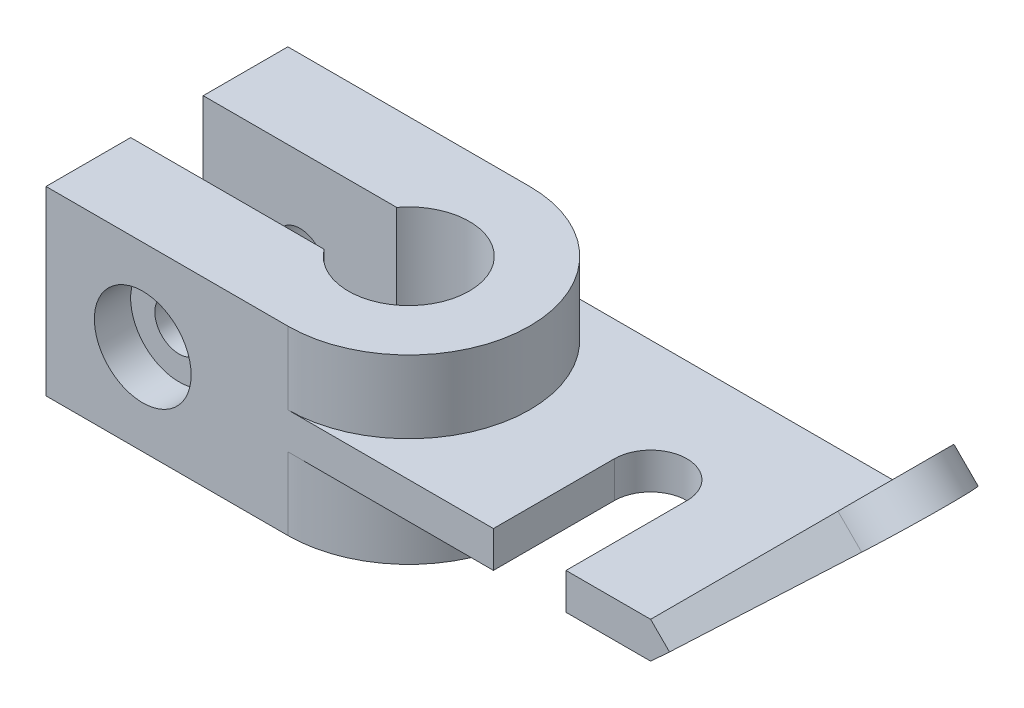
ISO-10303-21;
HEADER;
FILE_DESCRIPTION(('STEP AP214'),'2;1');
FILE_NAME('part.step','',(''),(''),'','','');
FILE_SCHEMA(('AUTOMOTIVE_DESIGN { 1 0 10303 214 1 1 1 1 }'));
ENDSEC;
DATA;
#1=APPLICATION_CONTEXT('core data for automotive mechanical design processes');
#2=APPLICATION_PROTOCOL_DEFINITION('international standard','automotive_design',2000,#1);
#3=PRODUCT_CONTEXT('',#1,'mechanical');
#4=PRODUCT('Part','Part','',(#3));
#5=PRODUCT_RELATED_PRODUCT_CATEGORY('part','',(#4));
#6=PRODUCT_DEFINITION_FORMATION('','',#4);
#7=PRODUCT_DEFINITION_CONTEXT('part definition',#1,'design');
#8=PRODUCT_DEFINITION('design','',#6,#7);
#9=PRODUCT_DEFINITION_SHAPE('','',#8);
#10=(LENGTH_UNIT() NAMED_UNIT(*) SI_UNIT(.MILLI.,.METRE.));
#11=(NAMED_UNIT(*) PLANE_ANGLE_UNIT() SI_UNIT($,.RADIAN.));
#12=(NAMED_UNIT(*) SI_UNIT($,.STERADIAN.) SOLID_ANGLE_UNIT());
#13=UNCERTAINTY_MEASURE_WITH_UNIT(LENGTH_MEASURE(1.E-05),#10,'distance_accuracy_value','');
#14=(GEOMETRIC_REPRESENTATION_CONTEXT(3) GLOBAL_UNCERTAINTY_ASSIGNED_CONTEXT((#13)) GLOBAL_UNIT_ASSIGNED_CONTEXT((#10,
#11,#12)) REPRESENTATION_CONTEXT('',''));
#15=CARTESIAN_POINT('',(0.,0.,0.));
#16=DIRECTION('',(0.,0.,1.));
#17=DIRECTION('',(1.,0.,0.));
#18=AXIS2_PLACEMENT_3D('',#15,#16,#17);
#19=CARTESIAN_POINT('',(-60.,22.5,30.));
#20=DIRECTION('',(0.,0.,-1.));
#21=DIRECTION('',(-1.,0.,0.));
#22=AXIS2_PLACEMENT_3D('',#19,#20,#21);
#23=PLANE('',#22);
#24=CARTESIAN_POINT('',(-36.,0.,30.));
#25=DIRECTION('',(0.,0.,1.));
#26=DIRECTION('',(1.,0.,0.));
#27=AXIS2_PLACEMENT_3D('',#24,#25,#26);
#28=CIRCLE('',#27,12.);
#29=CARTESIAN_POINT('',(-24.,0.,30.));
#30=VERTEX_POINT('',#29);
#31=EDGE_CURVE('E281',#30,#30,#28,.T.);
#32=ORIENTED_EDGE('',*,*,#31,.F.);
#33=EDGE_LOOP('',(#32));
#34=FACE_BOUND('',#33,.T.);
#35=DIRECTION('',(1.,0.,0.));
#36=VECTOR('',#35,1.);
#37=CARTESIAN_POINT('',(90.,-4.5,30.));
#38=LINE('',#37,#36);
#39=CARTESIAN_POINT('',(0.,-4.5,30.));
#40=VERTEX_POINT('',#39);
#41=CARTESIAN_POINT('',(51.,-4.5,30.));
#42=VERTEX_POINT('',#41);
#43=EDGE_CURVE('E253',#40,#42,#38,.T.);
#44=ORIENTED_EDGE('',*,*,#43,.T.);
#45=DIRECTION('',(0.,1.,0.));
#46=VECTOR('',#45,1.);
#47=CARTESIAN_POINT('',(51.,-4.5,30.));
#48=LINE('',#47,#46);
#49=CARTESIAN_POINT('',(51.,4.5,30.));
#50=VERTEX_POINT('',#49);
#51=EDGE_CURVE('E232',#42,#50,#48,.T.);
#52=ORIENTED_EDGE('',*,*,#51,.T.);
#53=DIRECTION('',(1.,0.,0.));
#54=VECTOR('',#53,1.);
#55=CARTESIAN_POINT('',(90.,4.5,30.));
#56=LINE('',#55,#54);
#57=CARTESIAN_POINT('',(0.,4.50000000000001,30.));
#58=VERTEX_POINT('',#57);
#59=EDGE_CURVE('E262',#58,#50,#56,.T.);
#60=ORIENTED_EDGE('',*,*,#59,.F.);
#61=DIRECTION('',(0.,-1.,0.));
#62=VECTOR('',#61,1.);
#63=CARTESIAN_POINT('',(0.,22.5,30.));
#64=LINE('',#63,#62);
#65=CARTESIAN_POINT('',(0.,22.5,30.));
#66=VERTEX_POINT('',#65);
#67=EDGE_CURVE('E324',#66,#58,#64,.T.);
#68=ORIENTED_EDGE('',*,*,#67,.F.);
#69=DIRECTION('',(1.,0.,0.));
#70=VECTOR('',#69,1.);
#71=CARTESIAN_POINT('',(-60.,22.5,30.));
#72=LINE('',#71,#70);
#73=CARTESIAN_POINT('',(-60.,22.5,30.));
#74=VERTEX_POINT('',#73);
#75=EDGE_CURVE('E307',#74,#66,#72,.T.);
#76=ORIENTED_EDGE('',*,*,#75,.F.);
#77=DIRECTION('',(0.,-1.,0.));
#78=VECTOR('',#77,1.);
#79=CARTESIAN_POINT('',(-60.,22.5,30.));
#80=LINE('',#79,#78);
#81=CARTESIAN_POINT('',(-60.,-22.5,30.));
#82=VERTEX_POINT('',#81);
#83=EDGE_CURVE('E330',#74,#82,#80,.T.);
#84=ORIENTED_EDGE('',*,*,#83,.T.);
#85=DIRECTION('',(1.,0.,0.));
#86=VECTOR('',#85,1.);
#87=CARTESIAN_POINT('',(-60.,-22.5,30.));
#88=LINE('',#87,#86);
#89=CARTESIAN_POINT('',(0.,-22.5,30.));
#90=VERTEX_POINT('',#89);
#91=EDGE_CURVE('E293',#82,#90,#88,.T.);
#92=ORIENTED_EDGE('',*,*,#91,.T.);
#93=EDGE_CURVE('E310',#40,#90,#64,.T.);
#94=ORIENTED_EDGE('',*,*,#93,.F.);
#95=EDGE_LOOP('',(#44,#52,#60,#68,#76,#84,#92,#94));
#96=FACE_BOUND('',#95,.T.);
#97=ADVANCED_FACE('F39',(#34,#96),#23,.F.);
#98=CARTESIAN_POINT('',(0.,22.5,0.));
#99=DIRECTION('',(0.,-1.,0.));
#100=DIRECTION('',(0.,0.,-1.));
#101=AXIS2_PLACEMENT_3D('',#98,#99,#100);
#102=CYLINDRICAL_SURFACE('',#101,30.);
#103=CARTESIAN_POINT('',(0.,-4.5,0.));
#104=DIRECTION('',(0.,-1.,0.));
#105=DIRECTION('',(0.,0.,1.));
#106=AXIS2_PLACEMENT_3D('',#103,#104,#105);
#107=CIRCLE('',#106,30.);
#108=CARTESIAN_POINT('',(0.,-4.49999999999999,-30.));
#109=VERTEX_POINT('',#108);
#110=EDGE_CURVE('E249',#109,#40,#107,.T.);
#111=ORIENTED_EDGE('',*,*,#110,.T.);
#112=ORIENTED_EDGE('',*,*,#93,.T.);
#113=CARTESIAN_POINT('',(0.,-22.5,0.));
#114=DIRECTION('',(0.,1.,0.));
#115=DIRECTION('',(0.,0.,1.));
#116=AXIS2_PLACEMENT_3D('',#113,#114,#115);
#117=CIRCLE('',#116,30.);
#118=CARTESIAN_POINT('',(0.,-22.5,-30.));
#119=VERTEX_POINT('',#118);
#120=EDGE_CURVE('E286',#90,#119,#117,.T.);
#121=ORIENTED_EDGE('',*,*,#120,.T.);
#122=DIRECTION('',(0.,-1.,0.));
#123=VECTOR('',#122,1.);
#124=CARTESIAN_POINT('',(0.,22.5,-30.));
#125=LINE('',#124,#123);
#126=EDGE_CURVE('E48',#109,#119,#125,.T.);
#127=ORIENTED_EDGE('',*,*,#126,.F.);
#128=EDGE_LOOP('',(#111,#112,#121,#127));
#129=FACE_BOUND('',#128,.T.);
#130=ADVANCED_FACE('F363',(#129),#102,.T.);
#131=CARTESIAN_POINT('',(-36.,0.,-54.));
#132=DIRECTION('',(0.,0.,1.));
#133=DIRECTION('',(1.,0.,0.));
#134=AXIS2_PLACEMENT_3D('',#131,#132,#133);
#135=CYLINDRICAL_SURFACE('',#134,6.);
#136=CARTESIAN_POINT('',(-36.,0.,-8.99999999999999));
#137=DIRECTION('',(0.,0.,-1.));
#138=DIRECTION('',(-1.,0.,0.));
#139=AXIS2_PLACEMENT_3D('',#136,#137,#138);
#140=CIRCLE('',#139,6.);
#141=CARTESIAN_POINT('',(-42.,0.,-8.99999999999999));
#142=VERTEX_POINT('',#141);
#143=EDGE_CURVE('E289',#142,#142,#140,.T.);
#144=ORIENTED_EDGE('',*,*,#143,.F.);
#145=EDGE_LOOP('',(#144));
#146=FACE_BOUND('',#145,.T.);
#147=CARTESIAN_POINT('',(-36.,0.,-21.));
#148=DIRECTION('',(0.,0.,-1.));
#149=DIRECTION('',(-1.,0.,0.));
#150=AXIS2_PLACEMENT_3D('',#147,#148,#149);
#151=CIRCLE('',#150,6.);
#152=CARTESIAN_POINT('',(-42.,0.,-21.));
#153=VERTEX_POINT('',#152);
#154=EDGE_CURVE('E43',#153,#153,#151,.F.);
#155=ORIENTED_EDGE('',*,*,#154,.F.);
#156=EDGE_LOOP('',(#155));
#157=FACE_BOUND('',#156,.T.);
#158=ADVANCED_FACE('F351',(#146,#157),#135,.F.);
#159=CARTESIAN_POINT('',(-36.,0.,9.00000000000001));
#160=DIRECTION('',(0.,0.,1.));
#161=DIRECTION('',(1.,0.,0.));
#162=AXIS2_PLACEMENT_3D('',#159,#160,#161);
#163=CIRCLE('',#162,6.);
#164=CARTESIAN_POINT('',(-30.,0.,9.00000000000001));
#165=VERTEX_POINT('',#164);
#166=EDGE_CURVE('E283',#165,#165,#163,.T.);
#167=ORIENTED_EDGE('',*,*,#166,.F.);
#168=EDGE_LOOP('',(#167));
#169=FACE_BOUND('',#168,.T.);
#170=CARTESIAN_POINT('',(-36.,0.,21.));
#171=DIRECTION('',(0.,0.,1.));
#172=DIRECTION('',(1.,0.,0.));
#173=AXIS2_PLACEMENT_3D('',#170,#171,#172);
#174=CIRCLE('',#173,6.);
#175=CARTESIAN_POINT('',(-30.,0.,21.));
#176=VERTEX_POINT('',#175);
#177=EDGE_CURVE('E278',#176,#176,#174,.F.);
#178=ORIENTED_EDGE('',*,*,#177,.F.);
#179=EDGE_LOOP('',(#178));
#180=FACE_BOUND('',#179,.T.);
#181=ADVANCED_FACE('F349',(#169,#180),#135,.F.);
#182=ORIENTED_EDGE('',*,*,#67,.T.);
#183=CARTESIAN_POINT('',(0.,4.5,0.));
#184=DIRECTION('',(0.,-1.,0.));
#185=DIRECTION('',(0.,0.,1.));
#186=AXIS2_PLACEMENT_3D('',#183,#184,#185);
#187=CIRCLE('',#186,30.);
#188=CARTESIAN_POINT('',(0.,4.50000000000001,-30.));
#189=VERTEX_POINT('',#188);
#190=EDGE_CURVE('E243',#189,#58,#187,.T.);
#191=ORIENTED_EDGE('',*,*,#190,.F.);
#192=CARTESIAN_POINT('',(0.,22.5,-30.));
#193=VERTEX_POINT('',#192);
#194=EDGE_CURVE('E11',#193,#189,#125,.T.);
#195=ORIENTED_EDGE('',*,*,#194,.F.);
#196=CARTESIAN_POINT('',(0.,22.5,0.));
#197=DIRECTION('',(0.,1.,0.));
#198=DIRECTION('',(0.,0.,1.));
#199=AXIS2_PLACEMENT_3D('',#196,#197,#198);
#200=CIRCLE('',#199,30.);
#201=EDGE_CURVE('E292',#66,#193,#200,.T.);
#202=ORIENTED_EDGE('',*,*,#201,.F.);
#203=EDGE_LOOP('',(#182,#191,#195,#202));
#204=FACE_BOUND('',#203,.T.);
#205=ADVANCED_FACE('F41',(#204),#102,.T.);
#206=CARTESIAN_POINT('',(0.,22.5,-30.));
#207=DIRECTION('',(0.,0.,1.));
#208=DIRECTION('',(1.,0.,0.));
#209=AXIS2_PLACEMENT_3D('',#206,#207,#208);
#210=PLANE('',#209);
#211=CARTESIAN_POINT('',(-36.,0.,-30.));
#212=DIRECTION('',(0.,0.,1.));
#213=DIRECTION('',(1.,0.,0.));
#214=AXIS2_PLACEMENT_3D('',#211,#212,#213);
#215=CIRCLE('',#214,12.);
#216=CARTESIAN_POINT('',(-24.,0.,-30.));
#217=VERTEX_POINT('',#216);
#218=EDGE_CURVE('E257',#217,#217,#215,.T.);
#219=ORIENTED_EDGE('',*,*,#218,.T.);
#220=EDGE_LOOP('',(#219));
#221=FACE_BOUND('',#220,.T.);
#222=DIRECTION('',(-1.,0.,0.));
#223=VECTOR('',#222,1.);
#224=CARTESIAN_POINT('',(0.,4.5,-30.));
#225=LINE('',#224,#223);
#226=CARTESIAN_POINT('',(90.,4.5,-30.));
#227=VERTEX_POINT('',#226);
#228=EDGE_CURVE('E246',#227,#189,#225,.T.);
#229=ORIENTED_EDGE('',*,*,#228,.F.);
#230=DIRECTION('',(-0.707106781186549,0.707106781186546,0.));
#231=VECTOR('',#230,1.);
#232=CARTESIAN_POINT('',(96.363961030679,-1.86396103067893,-30.));
#233=LINE('',#232,#231);
#234=CARTESIAN_POINT('',(94.6774076076125,-0.177407607612435,-30.));
#235=VERTEX_POINT('',#234);
#236=EDGE_CURVE('E183',#235,#227,#233,.T.);
#237=ORIENTED_EDGE('',*,*,#236,.F.);
#238=DIRECTION('',(-0.734413189883586,-0.678702634829876,0.));
#239=VECTOR('',#238,1.);
#240=CARTESIAN_POINT('',(139.143921292465,40.9159992311073,-30.));
#241=LINE('',#240,#239);
#242=CARTESIAN_POINT('',(90.,-4.5,-30.));
#243=VERTEX_POINT('',#242);
#244=EDGE_CURVE('E242',#235,#243,#241,.T.);
#245=ORIENTED_EDGE('',*,*,#244,.T.);
#246=DIRECTION('',(-1.,0.,0.));
#247=VECTOR('',#246,1.);
#248=CARTESIAN_POINT('',(0.,-4.5,-30.));
#249=LINE('',#248,#247);
#250=EDGE_CURVE('E260',#243,#109,#249,.T.);
#251=ORIENTED_EDGE('',*,*,#250,.T.);
#252=ORIENTED_EDGE('',*,*,#126,.T.);
#253=DIRECTION('',(-1.,0.,0.));
#254=VECTOR('',#253,1.);
#255=CARTESIAN_POINT('',(0.,-22.5,-30.));
#256=LINE('',#255,#254);
#257=CARTESIAN_POINT('',(-60.,-22.5,-30.));
#258=VERTEX_POINT('',#257);
#259=EDGE_CURVE('E313',#119,#258,#256,.T.);
#260=ORIENTED_EDGE('',*,*,#259,.T.);
#261=DIRECTION('',(0.,-1.,0.));
#262=VECTOR('',#261,1.);
#263=CARTESIAN_POINT('',(-60.,22.5,-30.));
#264=LINE('',#263,#262);
#265=CARTESIAN_POINT('',(-60.,22.5,-30.));
#266=VERTEX_POINT('',#265);
#267=EDGE_CURVE('E344',#266,#258,#264,.T.);
#268=ORIENTED_EDGE('',*,*,#267,.F.);
#269=DIRECTION('',(-1.,0.,0.));
#270=VECTOR('',#269,1.);
#271=CARTESIAN_POINT('',(0.,22.5,-30.));
#272=LINE('',#271,#270);
#273=EDGE_CURVE('E294',#193,#266,#272,.T.);
#274=ORIENTED_EDGE('',*,*,#273,.F.);
#275=ORIENTED_EDGE('',*,*,#194,.T.);
#276=EDGE_LOOP('',(#229,#237,#245,#251,#252,#260,#268,#274,#275));
#277=FACE_BOUND('',#276,.T.);
#278=ADVANCED_FACE('F360',(#221,#277),#210,.F.);
#279=CARTESIAN_POINT('',(-60.,22.5,-30.));
#280=DIRECTION('',(1.,0.,0.));
#281=DIRECTION('',(0.,0.,-1.));
#282=AXIS2_PLACEMENT_3D('',#279,#280,#281);
#283=PLANE('',#282);
#284=DIRECTION('',(0.,0.,1.));
#285=VECTOR('',#284,1.);
#286=CARTESIAN_POINT('',(-60.,-22.5,-30.));
#287=LINE('',#286,#285);
#288=CARTESIAN_POINT('',(-60.,-22.5,-8.99999999999999));
#289=VERTEX_POINT('',#288);
#290=EDGE_CURVE('E311',#258,#289,#287,.T.);
#291=ORIENTED_EDGE('',*,*,#290,.T.);
#292=DIRECTION('',(0.,-1.,0.));
#293=VECTOR('',#292,1.);
#294=CARTESIAN_POINT('',(-60.,22.5,-8.99999999999999));
#295=LINE('',#294,#293);
#296=CARTESIAN_POINT('',(-60.,22.5,-8.99999999999999));
#297=VERTEX_POINT('',#296);
#298=EDGE_CURVE('E338',#297,#289,#295,.T.);
#299=ORIENTED_EDGE('',*,*,#298,.F.);
#300=DIRECTION('',(0.,0.,1.));
#301=VECTOR('',#300,1.);
#302=CARTESIAN_POINT('',(-60.,22.5,-30.));
#303=LINE('',#302,#301);
#304=EDGE_CURVE('E297',#266,#297,#303,.T.);
#305=ORIENTED_EDGE('',*,*,#304,.F.);
#306=ORIENTED_EDGE('',*,*,#267,.T.);
#307=EDGE_LOOP('',(#291,#299,#305,#306));
#308=FACE_BOUND('',#307,.T.);
#309=ADVANCED_FACE('F491',(#308),#283,.F.);
#310=CARTESIAN_POINT('',(-12.,22.5,-8.99999999999999));
#311=DIRECTION('',(0.,0.,-1.));
#312=DIRECTION('',(-1.,0.,0.));
#313=AXIS2_PLACEMENT_3D('',#310,#311,#312);
#314=PLANE('',#313);
#315=ORIENTED_EDGE('',*,*,#143,.T.);
#316=EDGE_LOOP('',(#315));
#317=FACE_BOUND('',#316,.T.);
#318=DIRECTION('',(1.,0.,0.));
#319=VECTOR('',#318,1.);
#320=CARTESIAN_POINT('',(-12.,-22.5,-8.99999999999999));
#321=LINE('',#320,#319);
#322=CARTESIAN_POINT('',(-12.,-22.5,-8.99999999999999));
#323=VERTEX_POINT('',#322);
#324=EDGE_CURVE('E312',#289,#323,#321,.T.);
#325=ORIENTED_EDGE('',*,*,#324,.T.);
#326=DIRECTION('',(0.,-1.,0.));
#327=VECTOR('',#326,1.);
#328=CARTESIAN_POINT('',(-12.,22.5,-8.99999999999999));
#329=LINE('',#328,#327);
#330=CARTESIAN_POINT('',(-12.,22.5,-8.99999999999999));
#331=VERTEX_POINT('',#330);
#332=EDGE_CURVE('E336',#331,#323,#329,.T.);
#333=ORIENTED_EDGE('',*,*,#332,.F.);
#334=DIRECTION('',(1.,0.,0.));
#335=VECTOR('',#334,1.);
#336=CARTESIAN_POINT('',(-12.,22.5,-8.99999999999999));
#337=LINE('',#336,#335);
#338=EDGE_CURVE('E298',#297,#331,#337,.T.);
#339=ORIENTED_EDGE('',*,*,#338,.F.);
#340=ORIENTED_EDGE('',*,*,#298,.T.);
#341=EDGE_LOOP('',(#325,#333,#339,#340));
#342=FACE_BOUND('',#341,.T.);
#343=ADVANCED_FACE('F504',(#317,#342),#314,.F.);
#344=CARTESIAN_POINT('',(0.,22.5,0.));
#345=DIRECTION('',(0.,-1.,0.));
#346=DIRECTION('',(0.,0.,-1.));
#347=AXIS2_PLACEMENT_3D('',#344,#345,#346);
#348=CYLINDRICAL_SURFACE('',#347,15.);
#349=CARTESIAN_POINT('',(0.,-22.5,0.));
#350=DIRECTION('',(0.,-1.,0.));
#351=DIRECTION('',(0.,0.,1.));
#352=AXIS2_PLACEMENT_3D('',#349,#350,#351);
#353=CIRCLE('',#352,15.);
#354=CARTESIAN_POINT('',(-12.,-22.5,9.00000000000001));
#355=VERTEX_POINT('',#354);
#356=EDGE_CURVE('E320',#323,#355,#353,.T.);
#357=ORIENTED_EDGE('',*,*,#356,.T.);
#358=DIRECTION('',(0.,-1.,0.));
#359=VECTOR('',#358,1.);
#360=CARTESIAN_POINT('',(-12.,22.5,9.00000000000001));
#361=LINE('',#360,#359);
#362=CARTESIAN_POINT('',(-12.,22.5,9.00000000000001));
#363=VERTEX_POINT('',#362);
#364=EDGE_CURVE('E334',#363,#355,#361,.T.);
#365=ORIENTED_EDGE('',*,*,#364,.F.);
#366=CARTESIAN_POINT('',(0.,22.5,0.));
#367=DIRECTION('',(0.,-1.,0.));
#368=DIRECTION('',(0.,0.,1.));
#369=AXIS2_PLACEMENT_3D('',#366,#367,#368);
#370=CIRCLE('',#369,15.);
#371=EDGE_CURVE('E303',#331,#363,#370,.T.);
#372=ORIENTED_EDGE('',*,*,#371,.F.);
#373=ORIENTED_EDGE('',*,*,#332,.T.);
#374=EDGE_LOOP('',(#357,#365,#372,#373));
#375=FACE_BOUND('',#374,.T.);
#376=ADVANCED_FACE('F514',(#375),#348,.F.);
#377=CARTESIAN_POINT('',(-60.,22.5,9.00000000000001));
#378=DIRECTION('',(0.,0.,1.));
#379=DIRECTION('',(1.,0.,0.));
#380=AXIS2_PLACEMENT_3D('',#377,#378,#379);
#381=PLANE('',#380);
#382=ORIENTED_EDGE('',*,*,#166,.T.);
#383=EDGE_LOOP('',(#382));
#384=FACE_BOUND('',#383,.T.);
#385=DIRECTION('',(-1.,0.,0.));
#386=VECTOR('',#385,1.);
#387=CARTESIAN_POINT('',(-60.,-22.5,9.00000000000001));
#388=LINE('',#387,#386);
#389=CARTESIAN_POINT('',(-60.,-22.5,9.00000000000001));
#390=VERTEX_POINT('',#389);
#391=EDGE_CURVE('E317',#355,#390,#388,.T.);
#392=ORIENTED_EDGE('',*,*,#391,.T.);
#393=DIRECTION('',(0.,-1.,0.));
#394=VECTOR('',#393,1.);
#395=CARTESIAN_POINT('',(-60.,22.5,9.00000000000001));
#396=LINE('',#395,#394);
#397=CARTESIAN_POINT('',(-60.,22.5,9.00000000000001));
#398=VERTEX_POINT('',#397);
#399=EDGE_CURVE('E329',#398,#390,#396,.T.);
#400=ORIENTED_EDGE('',*,*,#399,.F.);
#401=DIRECTION('',(-1.,0.,0.));
#402=VECTOR('',#401,1.);
#403=CARTESIAN_POINT('',(-60.,22.5,9.00000000000001));
#404=LINE('',#403,#402);
#405=EDGE_CURVE('E302',#363,#398,#404,.T.);
#406=ORIENTED_EDGE('',*,*,#405,.F.);
#407=ORIENTED_EDGE('',*,*,#364,.T.);
#408=EDGE_LOOP('',(#392,#400,#406,#407));
#409=FACE_BOUND('',#408,.T.);
#410=ADVANCED_FACE('F391',(#384,#409),#381,.F.);
#411=CARTESIAN_POINT('',(-60.,22.5,9.00000000000001));
#412=DIRECTION('',(1.,0.,0.));
#413=DIRECTION('',(0.,0.,-1.));
#414=AXIS2_PLACEMENT_3D('',#411,#412,#413);
#415=PLANE('',#414);
#416=DIRECTION('',(0.,0.,1.));
#417=VECTOR('',#416,1.);
#418=CARTESIAN_POINT('',(-60.,-22.5,9.00000000000001));
#419=LINE('',#418,#417);
#420=EDGE_CURVE('E321',#390,#82,#419,.T.);
#421=ORIENTED_EDGE('',*,*,#420,.T.);
#422=ORIENTED_EDGE('',*,*,#83,.F.);
#423=DIRECTION('',(0.,0.,1.));
#424=VECTOR('',#423,1.);
#425=CARTESIAN_POINT('',(-60.,22.5,9.00000000000001));
#426=LINE('',#425,#424);
#427=EDGE_CURVE('E301',#398,#74,#426,.T.);
#428=ORIENTED_EDGE('',*,*,#427,.F.);
#429=ORIENTED_EDGE('',*,*,#399,.T.);
#430=EDGE_LOOP('',(#421,#422,#428,#429));
#431=FACE_BOUND('',#430,.T.);
#432=ADVANCED_FACE('F381',(#431),#415,.F.);
#433=DIRECTION('',(0.734413189883586,0.678702634829876,0.));
#434=VECTOR('',#433,1.);
#435=CARTESIAN_POINT('',(139.143921292465,40.9159992311073,30.));
#436=LINE('',#435,#434);
#437=CARTESIAN_POINT('',(90.,-4.5,30.));
#438=VERTEX_POINT('',#437);
#439=CARTESIAN_POINT('',(94.6774076076125,-0.177407607612432,30.));
#440=VERTEX_POINT('',#439);
#441=EDGE_CURVE('E237',#438,#440,#436,.T.);
#442=ORIENTED_EDGE('',*,*,#441,.T.);
#443=DIRECTION('',(-0.707106781186549,0.707106781186546,0.));
#444=VECTOR('',#443,1.);
#445=CARTESIAN_POINT('',(96.363961030679,-1.86396103067893,30.));
#446=LINE('',#445,#444);
#447=CARTESIAN_POINT('',(90.,4.49999999999999,30.));
#448=VERTEX_POINT('',#447);
#449=EDGE_CURVE('E203',#440,#448,#446,.T.);
#450=ORIENTED_EDGE('',*,*,#449,.T.);
#451=CARTESIAN_POINT('',(69.,4.5,30.));
#452=VERTEX_POINT('',#451);
#453=EDGE_CURVE('E263',#452,#448,#56,.T.);
#454=ORIENTED_EDGE('',*,*,#453,.F.);
#455=DIRECTION('',(0.,1.,0.));
#456=VECTOR('',#455,1.);
#457=CARTESIAN_POINT('',(69.,-4.5,30.));
#458=LINE('',#457,#456);
#459=CARTESIAN_POINT('',(69.,-4.5,30.));
#460=VERTEX_POINT('',#459);
#461=EDGE_CURVE('E57',#460,#452,#458,.T.);
#462=ORIENTED_EDGE('',*,*,#461,.F.);
#463=EDGE_CURVE('E250',#460,#438,#38,.T.);
#464=ORIENTED_EDGE('',*,*,#463,.T.);
#465=EDGE_LOOP('',(#442,#450,#454,#462,#464));
#466=FACE_BOUND('',#465,.T.);
#467=ADVANCED_FACE('F367',(#466),#23,.F.);
#468=CARTESIAN_POINT('',(0.,22.5,0.));
#469=DIRECTION('',(0.,1.,0.));
#470=DIRECTION('',(0.,0.,1.));
#471=AXIS2_PLACEMENT_3D('',#468,#469,#470);
#472=PLANE('',#471);
#473=ORIENTED_EDGE('',*,*,#201,.T.);
#474=ORIENTED_EDGE('',*,*,#273,.T.);
#475=ORIENTED_EDGE('',*,*,#304,.T.);
#476=ORIENTED_EDGE('',*,*,#338,.T.);
#477=ORIENTED_EDGE('',*,*,#371,.T.);
#478=ORIENTED_EDGE('',*,*,#405,.T.);
#479=ORIENTED_EDGE('',*,*,#427,.T.);
#480=ORIENTED_EDGE('',*,*,#75,.T.);
#481=EDGE_LOOP('',(#473,#474,#475,#476,#477,#478,#479,#480));
#482=FACE_BOUND('',#481,.T.);
#483=ADVANCED_FACE('F379',(#482),#472,.T.);
#484=CARTESIAN_POINT('',(0.,-22.5,0.));
#485=DIRECTION('',(0.,1.,0.));
#486=DIRECTION('',(0.,0.,1.));
#487=AXIS2_PLACEMENT_3D('',#484,#485,#486);
#488=PLANE('',#487);
#489=ORIENTED_EDGE('',*,*,#120,.F.);
#490=ORIENTED_EDGE('',*,*,#91,.F.);
#491=ORIENTED_EDGE('',*,*,#420,.F.);
#492=ORIENTED_EDGE('',*,*,#391,.F.);
#493=ORIENTED_EDGE('',*,*,#356,.F.);
#494=ORIENTED_EDGE('',*,*,#324,.F.);
#495=ORIENTED_EDGE('',*,*,#290,.F.);
#496=ORIENTED_EDGE('',*,*,#259,.F.);
#497=EDGE_LOOP('',(#489,#490,#491,#492,#493,#494,#495,#496));
#498=FACE_BOUND('',#497,.T.);
#499=ADVANCED_FACE('F389',(#498),#488,.F.);
#500=CARTESIAN_POINT('',(-36.,0.,21.));
#501=DIRECTION('',(0.,0.,1.));
#502=DIRECTION('',(1.,0.,0.));
#503=AXIS2_PLACEMENT_3D('',#500,#501,#502);
#504=PLANE('',#503);
#505=CARTESIAN_POINT('',(-36.,0.,21.));
#506=DIRECTION('',(0.,0.,1.));
#507=DIRECTION('',(1.,0.,0.));
#508=AXIS2_PLACEMENT_3D('',#505,#506,#507);
#509=CIRCLE('',#508,12.);
#510=CARTESIAN_POINT('',(-24.,0.,21.));
#511=VERTEX_POINT('',#510);
#512=EDGE_CURVE('E280',#511,#511,#509,.T.);
#513=ORIENTED_EDGE('',*,*,#512,.T.);
#514=EDGE_LOOP('',(#513));
#515=FACE_BOUND('',#514,.T.);
#516=ORIENTED_EDGE('',*,*,#177,.T.);
#517=EDGE_LOOP('',(#516));
#518=FACE_BOUND('',#517,.T.);
#519=ADVANCED_FACE('F350',(#515,#518),#504,.T.);
#520=CARTESIAN_POINT('',(-36.,0.,21.));
#521=DIRECTION('',(0.,0.,1.));
#522=DIRECTION('',(1.,0.,0.));
#523=AXIS2_PLACEMENT_3D('',#520,#521,#522);
#524=CYLINDRICAL_SURFACE('',#523,12.);
#525=ORIENTED_EDGE('',*,*,#512,.F.);
#526=EDGE_LOOP('',(#525));
#527=FACE_BOUND('',#526,.T.);
#528=ORIENTED_EDGE('',*,*,#31,.T.);
#529=EDGE_LOOP('',(#528));
#530=FACE_BOUND('',#529,.T.);
#531=ADVANCED_FACE('F444',(#527,#530),#524,.F.);
#532=CARTESIAN_POINT('',(-36.,0.,-21.));
#533=DIRECTION('',(0.,0.,-1.));
#534=DIRECTION('',(1.,0.,0.));
#535=AXIS2_PLACEMENT_3D('',#532,#533,#534);
#536=PLANE('',#535);
#537=CARTESIAN_POINT('',(-36.,0.,-21.));
#538=DIRECTION('',(0.,0.,1.));
#539=DIRECTION('',(1.,0.,0.));
#540=AXIS2_PLACEMENT_3D('',#537,#538,#539);
#541=CIRCLE('',#540,12.);
#542=CARTESIAN_POINT('',(-24.,0.,-21.));
#543=VERTEX_POINT('',#542);
#544=EDGE_CURVE('E275',#543,#543,#541,.T.);
#545=ORIENTED_EDGE('',*,*,#544,.F.);
#546=EDGE_LOOP('',(#545));
#547=FACE_BOUND('',#546,.T.);
#548=ORIENTED_EDGE('',*,*,#154,.T.);
#549=EDGE_LOOP('',(#548));
#550=FACE_BOUND('',#549,.T.);
#551=ADVANCED_FACE('F439',(#547,#550),#536,.T.);
#552=CARTESIAN_POINT('',(-36.,0.,-21.));
#553=DIRECTION('',(0.,0.,-1.));
#554=DIRECTION('',(-1.,0.,0.));
#555=AXIS2_PLACEMENT_3D('',#552,#553,#554);
#556=CYLINDRICAL_SURFACE('',#555,12.);
#557=ORIENTED_EDGE('',*,*,#544,.T.);
#558=EDGE_LOOP('',(#557));
#559=FACE_BOUND('',#558,.T.);
#560=ORIENTED_EDGE('',*,*,#218,.F.);
#561=EDGE_LOOP('',(#560));
#562=FACE_BOUND('',#561,.T.);
#563=ADVANCED_FACE('F436',(#559,#562),#556,.F.);
#564=CARTESIAN_POINT('',(0.,-4.5,0.));
#565=DIRECTION('',(0.,1.,0.));
#566=DIRECTION('',(0.,0.,1.));
#567=AXIS2_PLACEMENT_3D('',#564,#565,#566);
#568=PLANE('',#567);
#569=CARTESIAN_POINT('',(60.,-4.5,0.));
#570=DIRECTION('',(0.,1.,0.));
#571=DIRECTION('',(0.,0.,-1.));
#572=AXIS2_PLACEMENT_3D('',#569,#570,#571);
#573=CIRCLE('',#572,9.);
#574=CARTESIAN_POINT('',(69.,-4.5,0.));
#575=VERTEX_POINT('',#574);
#576=CARTESIAN_POINT('',(51.,-4.5,0.));
#577=VERTEX_POINT('',#576);
#578=EDGE_CURVE('E222',#575,#577,#573,.T.);
#579=ORIENTED_EDGE('',*,*,#578,.T.);
#580=DIRECTION('',(0.,0.,1.));
#581=VECTOR('',#580,1.);
#582=CARTESIAN_POINT('',(51.,-4.5,30.));
#583=LINE('',#582,#581);
#584=EDGE_CURVE('E223',#577,#42,#583,.T.);
#585=ORIENTED_EDGE('',*,*,#584,.T.);
#586=ORIENTED_EDGE('',*,*,#43,.F.);
#587=ORIENTED_EDGE('',*,*,#110,.F.);
#588=ORIENTED_EDGE('',*,*,#250,.F.);
#589=DIRECTION('',(0.,0.,-1.));
#590=VECTOR('',#589,1.);
#591=CARTESIAN_POINT('',(90.,-4.5,-30.));
#592=LINE('',#591,#590);
#593=EDGE_CURVE('E255',#438,#243,#592,.T.);
#594=ORIENTED_EDGE('',*,*,#593,.F.);
#595=ORIENTED_EDGE('',*,*,#463,.F.);
#596=DIRECTION('',(0.,0.,-1.));
#597=VECTOR('',#596,1.);
#598=CARTESIAN_POINT('',(69.,-4.5,0.));
#599=LINE('',#598,#597);
#600=EDGE_CURVE('E217',#460,#575,#599,.T.);
#601=ORIENTED_EDGE('',*,*,#600,.T.);
#602=EDGE_LOOP('',(#579,#585,#586,#587,#588,#594,#595,#601));
#603=FACE_BOUND('',#602,.T.);
#604=ADVANCED_FACE('F432',(#603),#568,.F.);
#605=CARTESIAN_POINT('',(0.,4.5,0.));
#606=DIRECTION('',(0.,1.,0.));
#607=DIRECTION('',(0.,0.,1.));
#608=AXIS2_PLACEMENT_3D('',#605,#606,#607);
#609=PLANE('',#608);
#610=DIRECTION('',(0.,0.,1.));
#611=VECTOR('',#610,1.);
#612=CARTESIAN_POINT('',(51.,4.5,30.));
#613=LINE('',#612,#611);
#614=CARTESIAN_POINT('',(51.,4.5,0.));
#615=VERTEX_POINT('',#614);
#616=EDGE_CURVE('E225',#615,#50,#613,.T.);
#617=ORIENTED_EDGE('',*,*,#616,.F.);
#618=CARTESIAN_POINT('',(60.,4.5,0.));
#619=DIRECTION('',(0.,1.,0.));
#620=DIRECTION('',(0.,0.,-1.));
#621=AXIS2_PLACEMENT_3D('',#618,#619,#620);
#622=CIRCLE('',#621,9.);
#623=CARTESIAN_POINT('',(69.,4.5,0.));
#624=VERTEX_POINT('',#623);
#625=EDGE_CURVE('E228',#624,#615,#622,.T.);
#626=ORIENTED_EDGE('',*,*,#625,.F.);
#627=DIRECTION('',(0.,0.,-1.));
#628=VECTOR('',#627,1.);
#629=CARTESIAN_POINT('',(69.,4.5,0.));
#630=LINE('',#629,#628);
#631=EDGE_CURVE('E220',#452,#624,#630,.T.);
#632=ORIENTED_EDGE('',*,*,#631,.F.);
#633=ORIENTED_EDGE('',*,*,#453,.T.);
#634=DIRECTION('',(0.,0.,-1.));
#635=VECTOR('',#634,1.);
#636=CARTESIAN_POINT('',(90.,4.5,-30.));
#637=LINE('',#636,#635);
#638=EDGE_CURVE('E270',#448,#227,#637,.T.);
#639=ORIENTED_EDGE('',*,*,#638,.T.);
#640=ORIENTED_EDGE('',*,*,#228,.T.);
#641=ORIENTED_EDGE('',*,*,#190,.T.);
#642=ORIENTED_EDGE('',*,*,#59,.T.);
#643=EDGE_LOOP('',(#617,#626,#632,#633,#639,#640,#641,#642));
#644=FACE_BOUND('',#643,.T.);
#645=ADVANCED_FACE('F433',(#644),#609,.T.);
#646=CARTESIAN_POINT('',(139.143921292465,40.9159992311073,-101.388299354391));
#647=DIRECTION('',(0.678702634829876,-0.734413189883586,0.));
#648=DIRECTION('',(0.734413189883586,0.678702634829876,0.));
#649=AXIS2_PLACEMENT_3D('',#646,#647,#648);
#650=PLANE('',#649);
#651=DIRECTION('',(0.689121133653438,0.636846308821982,-0.34574389668079));
#652=VECTOR('',#651,1.);
#653=CARTESIAN_POINT('',(165.132946526525,64.9335688308753,-5.34875275036981));
#654=LINE('',#653,#652);
#655=CARTESIAN_POINT('',(126.42113673388,29.1583299500679,14.0736264390714));
#656=VERTEX_POINT('',#655);
#657=EDGE_CURVE('E214',#440,#656,#654,.T.);
#658=ORIENTED_EDGE('',*,*,#657,.F.);
#659=ORIENTED_EDGE('',*,*,#441,.F.);
#660=ORIENTED_EDGE('',*,*,#593,.T.);
#661=ORIENTED_EDGE('',*,*,#244,.F.);
#662=DIRECTION('',(-0.689121133653438,-0.636846308821982,-0.34574389668079));
#663=VECTOR('',#662,1.);
#664=CARTESIAN_POINT('',(116.819510504958,20.2850565530392,-18.8909270626356));
#665=LINE('',#664,#663);
#666=CARTESIAN_POINT('',(126.42113673388,29.1583299500679,-14.0736264390714));
#667=VERTEX_POINT('',#666);
#668=EDGE_CURVE('E215',#667,#235,#665,.T.);
#669=ORIENTED_EDGE('',*,*,#668,.F.);
#670=CARTESIAN_POINT('',(122.606788103883,25.6333272662942,0.));
#671=DIRECTION('',(0.678702634829876,-0.734413189883586,0.));
#672=DIRECTION('',(-0.734413189883586,-0.678702634829876,0.));
#673=AXIS2_PLACEMENT_3D('',#670,#671,#672);
#674=ELLIPSE('',#673,15.0116523108768,15.);
#675=EDGE_CURVE('E182',#656,#667,#674,.F.);
#676=ORIENTED_EDGE('',*,*,#675,.F.);
#677=EDGE_LOOP('',(#658,#659,#660,#661,#669,#676));
#678=FACE_BOUND('',#677,.T.);
#679=CARTESIAN_POINT('',(122.606788103883,25.6333272662942,0.));
#680=DIRECTION('',(0.678702634829876,-0.734413189883586,0.));
#681=DIRECTION('',(-0.734413189883586,-0.678702634829876,0.));
#682=AXIS2_PLACEMENT_3D('',#679,#680,#681);
#683=ELLIPSE('',#682,7.50582615543841,7.50000000000001);
#684=CARTESIAN_POINT('',(117.094410374356,20.5391032780231,0.));
#685=VERTEX_POINT('',#684);
#686=EDGE_CURVE('E207',#685,#685,#683,.T.);
#687=ORIENTED_EDGE('',*,*,#686,.F.);
#688=EDGE_LOOP('',(#687));
#689=FACE_BOUND('',#688,.T.);
#690=ADVANCED_FACE('F396',(#678,#689),#650,.T.);
#691=CARTESIAN_POINT('',(90.,4.5,-101.388299354391));
#692=DIRECTION('',(-0.707106781186549,0.707106781186546,0.));
#693=DIRECTION('',(-0.707106781186546,-0.707106781186549,0.));
#694=AXIS2_PLACEMENT_3D('',#691,#692,#693);
#695=PLANE('',#694);
#696=DIRECTION('',(-0.663437112730243,-0.663437112730245,0.345980338898493));
#697=VECTOR('',#696,1.);
#698=CARTESIAN_POINT('',(90.,4.49999999999999,30.));
#699=LINE('',#698,#697);
#700=CARTESIAN_POINT('',(120.539733341974,35.039733341974,14.0736264390714));
#701=VERTEX_POINT('',#700);
#702=EDGE_CURVE('E197',#701,#448,#699,.T.);
#703=ORIENTED_EDGE('',*,*,#702,.F.);
#704=CARTESIAN_POINT('',(116.870057685089,31.3700576850888,0.));
#705=DIRECTION('',(0.707106781186549,-0.707106781186546,0.));
#706=DIRECTION('',(-0.707106781186546,-0.707106781186549,0.));
#707=AXIS2_PLACEMENT_3D('',#704,#705,#706);
#708=CIRCLE('',#707,15.);
#709=CARTESIAN_POINT('',(120.539733341974,35.039733341974,-14.0736264390714));
#710=VERTEX_POINT('',#709);
#711=EDGE_CURVE('E177',#710,#701,#708,.T.);
#712=ORIENTED_EDGE('',*,*,#711,.F.);
#713=DIRECTION('',(0.663437112730242,0.663437112730245,0.345980338898493));
#714=VECTOR('',#713,1.);
#715=CARTESIAN_POINT('',(90.,4.49999999999999,-30.));
#716=LINE('',#715,#714);
#717=EDGE_CURVE('E189',#227,#710,#716,.T.);
#718=ORIENTED_EDGE('',*,*,#717,.F.);
#719=ORIENTED_EDGE('',*,*,#638,.F.);
#720=EDGE_LOOP('',(#703,#712,#718,#719));
#721=FACE_BOUND('',#720,.T.);
#722=CARTESIAN_POINT('',(116.870057685089,31.3700576850888,0.));
#723=DIRECTION('',(-0.707106781186549,0.707106781186546,0.));
#724=DIRECTION('',(-0.707106781186546,-0.707106781186549,0.));
#725=AXIS2_PLACEMENT_3D('',#722,#723,#724);
#726=CIRCLE('',#725,7.50000000000001);
#727=CARTESIAN_POINT('',(111.56675682619,26.0667568261897,0.));
#728=VERTEX_POINT('',#727);
#729=EDGE_CURVE('E204',#728,#728,#726,.T.);
#730=ORIENTED_EDGE('',*,*,#729,.F.);
#731=EDGE_LOOP('',(#730));
#732=FACE_BOUND('',#731,.T.);
#733=ADVANCED_FACE('F191',(#721,#732),#695,.T.);
#734=CARTESIAN_POINT('',(51.,-4.5,30.));
#735=DIRECTION('',(-1.,0.,0.));
#736=DIRECTION('',(0.,0.,1.));
#737=AXIS2_PLACEMENT_3D('',#734,#735,#736);
#738=PLANE('',#737);
#739=ORIENTED_EDGE('',*,*,#616,.T.);
#740=ORIENTED_EDGE('',*,*,#51,.F.);
#741=ORIENTED_EDGE('',*,*,#584,.F.);
#742=DIRECTION('',(0.,1.,0.));
#743=VECTOR('',#742,1.);
#744=CARTESIAN_POINT('',(51.,-4.5,0.));
#745=LINE('',#744,#743);
#746=EDGE_CURVE('E240',#577,#615,#745,.T.);
#747=ORIENTED_EDGE('',*,*,#746,.T.);
#748=EDGE_LOOP('',(#739,#740,#741,#747));
#749=FACE_BOUND('',#748,.T.);
#750=ADVANCED_FACE('F420',(#749),#738,.F.);
#751=CARTESIAN_POINT('',(60.,-4.5,0.));
#752=DIRECTION('',(0.,1.,0.));
#753=DIRECTION('',(0.,0.,1.));
#754=AXIS2_PLACEMENT_3D('',#751,#752,#753);
#755=CYLINDRICAL_SURFACE('',#754,9.);
#756=ORIENTED_EDGE('',*,*,#625,.T.);
#757=ORIENTED_EDGE('',*,*,#746,.F.);
#758=ORIENTED_EDGE('',*,*,#578,.F.);
#759=DIRECTION('',(0.,1.,0.));
#760=VECTOR('',#759,1.);
#761=CARTESIAN_POINT('',(69.,-4.5,0.));
#762=LINE('',#761,#760);
#763=EDGE_CURVE('E239',#575,#624,#762,.T.);
#764=ORIENTED_EDGE('',*,*,#763,.T.);
#765=EDGE_LOOP('',(#756,#757,#758,#764));
#766=FACE_BOUND('',#765,.T.);
#767=ADVANCED_FACE('F425',(#766),#755,.F.);
#768=CARTESIAN_POINT('',(69.,-4.5,0.));
#769=DIRECTION('',(1.,0.,0.));
#770=DIRECTION('',(0.,0.,-1.));
#771=AXIS2_PLACEMENT_3D('',#768,#769,#770);
#772=PLANE('',#771);
#773=ORIENTED_EDGE('',*,*,#631,.T.);
#774=ORIENTED_EDGE('',*,*,#763,.F.);
#775=ORIENTED_EDGE('',*,*,#600,.F.);
#776=ORIENTED_EDGE('',*,*,#461,.T.);
#777=EDGE_LOOP('',(#773,#774,#775,#776));
#778=FACE_BOUND('',#777,.T.);
#779=ADVANCED_FACE('F412',(#778),#772,.F.);
#780=CARTESIAN_POINT('',(123.234018715768,25.0060966544099,0.));
#781=DIRECTION('',(-0.707106781186549,0.707106781186546,0.));
#782=DIRECTION('',(-0.707106781186546,-0.707106781186549,0.));
#783=AXIS2_PLACEMENT_3D('',#780,#781,#782);
#784=CYLINDRICAL_SURFACE('',#783,7.50000000000001);
#785=ORIENTED_EDGE('',*,*,#686,.T.);
#786=EDGE_LOOP('',(#785));
#787=FACE_BOUND('',#786,.T.);
#788=ORIENTED_EDGE('',*,*,#729,.T.);
#789=EDGE_LOOP('',(#788));
#790=FACE_BOUND('',#789,.T.);
#791=ADVANCED_FACE('F406',(#787,#790),#784,.F.);
#792=CARTESIAN_POINT('',(96.363961030679,-1.86396103067893,30.));
#793=DIRECTION('',(-0.244645043792344,-0.244645043792345,-0.938241762604758));
#794=DIRECTION('',(0.,0.967645901653553,-0.252312126171302));
#795=AXIS2_PLACEMENT_3D('',#792,#793,#794);
#796=PLANE('',#795);
#797=ORIENTED_EDGE('',*,*,#657,.T.);
#798=DIRECTION('',(-0.707106781186549,0.707106781186546,0.));
#799=VECTOR('',#798,1.);
#800=CARTESIAN_POINT('',(126.903694372653,28.6757723112951,14.0736264390714));
#801=LINE('',#800,#799);
#802=EDGE_CURVE('E184',#656,#701,#801,.T.);
#803=ORIENTED_EDGE('',*,*,#802,.T.);
#804=ORIENTED_EDGE('',*,*,#702,.T.);
#805=ORIENTED_EDGE('',*,*,#449,.F.);
#806=EDGE_LOOP('',(#797,#803,#804,#805));
#807=FACE_BOUND('',#806,.T.);
#808=ADVANCED_FACE('F404',(#807),#796,.F.);
#809=CARTESIAN_POINT('',(123.234018715768,25.0060966544099,0.));
#810=DIRECTION('',(-0.707106781186549,0.707106781186546,0.));
#811=DIRECTION('',(-0.707106781186546,-0.707106781186549,0.));
#812=AXIS2_PLACEMENT_3D('',#809,#810,#811);
#813=CYLINDRICAL_SURFACE('',#812,15.);
#814=ORIENTED_EDGE('',*,*,#675,.T.);
#815=DIRECTION('',(-0.707106781186549,0.707106781186546,0.));
#816=VECTOR('',#815,1.);
#817=CARTESIAN_POINT('',(126.903694372653,28.6757723112951,-14.0736264390714));
#818=LINE('',#817,#816);
#819=EDGE_CURVE('E174',#667,#710,#818,.T.);
#820=ORIENTED_EDGE('',*,*,#819,.T.);
#821=ORIENTED_EDGE('',*,*,#711,.T.);
#822=ORIENTED_EDGE('',*,*,#802,.F.);
#823=EDGE_LOOP('',(#814,#820,#821,#822));
#824=FACE_BOUND('',#823,.T.);
#825=ADVANCED_FACE('F175',(#824),#813,.T.);
#826=CARTESIAN_POINT('',(96.363961030679,-1.86396103067893,-30.));
#827=DIRECTION('',(-0.244645043792344,-0.244645043792345,0.938241762604758));
#828=DIRECTION('',(0.,-0.967645901653553,-0.252312126171302));
#829=AXIS2_PLACEMENT_3D('',#826,#827,#828);
#830=PLANE('',#829);
#831=ORIENTED_EDGE('',*,*,#668,.T.);
#832=ORIENTED_EDGE('',*,*,#236,.T.);
#833=ORIENTED_EDGE('',*,*,#717,.T.);
#834=ORIENTED_EDGE('',*,*,#819,.F.);
#835=EDGE_LOOP('',(#831,#832,#833,#834));
#836=FACE_BOUND('',#835,.T.);
#837=ADVANCED_FACE('F188',(#836),#830,.F.);
#838=CLOSED_SHELL('',(#97,#130,#158,#181,#205,#278,#309,#343,#376,#410,#432,#467,#483,#499,#519,
#531,#551,#563,#604,#645,#690,#733,#750,#767,#779,#791,#808,#825,#837));
#839=MANIFOLD_SOLID_BREP('B2',#838);
#840=ADVANCED_BREP_SHAPE_REPRESENTATION('',(#18,#839),#14);
#841=SHAPE_DEFINITION_REPRESENTATION(#9,#840);
ENDSEC;
END-ISO-10303-21;
